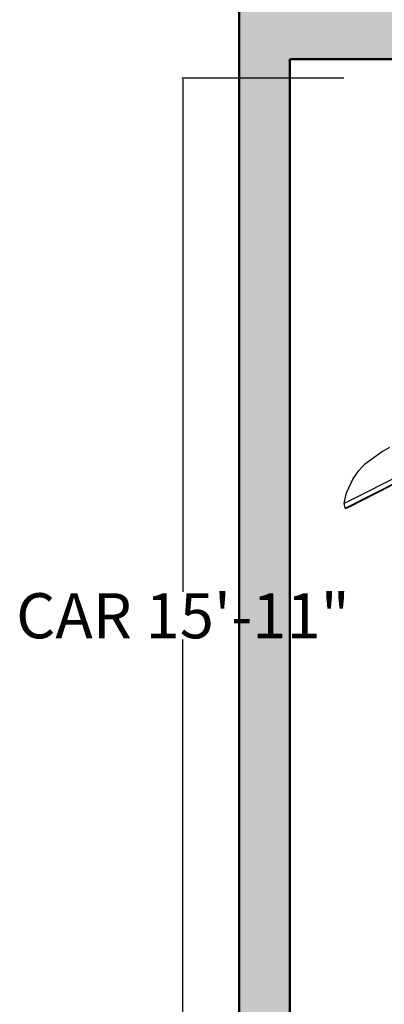
# Model space of a CAD drawing. Units: inches. Extents: x 22042254 to 25404563, y 17568978 to 17626777.
# Tile 25 of 45: x 22179745 to 22179810, y 17626227 to 17626402. Entities that reach past the tile are written whole.
import ezdxf

# ---------------------------------------------------------------- set-up
doc = ezdxf.new("R2010")
doc.units = ezdxf.units.IN
doc.header["$MEASUREMENT"] = 0
for name, color, linetype, lineweight in [('A-ANNO-DIMS', 2, 'Continuous', 18), ('A-SITE-VEHI', 8, 'Continuous', 18), ('A-WALL-PATT', 244, 'Continuous', 13), ('walls', 252, 'Continuous', 50)]:
    doc.layers.add(name, color=color, linetype=linetype, lineweight=lineweight)
doc.layers.add('Edges', color=250, linetype='Continuous')
doc.styles.get("Standard").update_dxf_attribs({"font": 'arial.ttf'})
doc.dimstyles.get("Standard").update_dxf_attribs({"dimtxt": 8, "dimasz": 0.18, "dimexe": 0.18, "dimexo": 0.0625, "dimgap": 0.09, "dimtad": 0, "dimtih": 1, "dimtoh": 1, "dimzin": 0, "dimdsep": 46, "dimlunit": 3, "dimtxsty": 'Standard', "dimcen": 0.09, "dimadec": 0, "dimazin": 0, "dimtfac": 1, "dimtofl": 0, "dimtmove": 0, "dimatfit": 3, "dimfxl": 1, "dimtolj": 1, "dimtzin": 0, "dimarcsym": 0})

# ---------------------------------------------------------------- blocks, each defined once
blk = doc.blocks.new('Nissan Qashqai pl')
at = {"layer": 'Edges'}
for p, q in [((8.8918, 11.0997), (9.0186, 10.8486)), ((9.0333, 10.8597), (8.9232, 11.0779)), ((9.0386, 10.8534), (8.9254, 11.0778)), ((8.9483, 11.0359), (9.0343, 10.8656)), ((8.7908, 11.0322), (8.8066, 11.0041)), ((8.8066, 11.0041), (8.8591, 10.9315)), ((8.8591, 10.9315), (8.8879, 10.9041)), ((8.8885, 10.9037), (8.8879, 10.9041)), ((8.8885, 10.9037), (8.9173, 10.8831)), ((8.9173, 10.8831), (8.9731, 10.8577)), ((9.0186, 10.8486), (8.9731, 10.8577)), ((9.0374, 10.8517), (9.0186, 10.8486)), ((9.0356, 10.8553), (9.0333, 10.8597)), ((9.0343, 10.8656), (9.0347, 10.8648)), ((9.0347, 10.8648), (9.0362, 10.8619)), ((9.0356, 10.8553), (9.0374, 10.8517)), ((9.0362, 10.8619), (9.037, 10.8603)), ((9.0371, 10.8601), (9.037, 10.8603)), ((9.0371, 10.8601), (9.0376, 10.8591)), ((9.0376, 10.8591), (9.0371, 10.8595)), ((9.0386, 10.8534), (9.0374, 10.8517)), ((9.0376, 10.8591), (9.0386, 10.8534))]:
    blk.add_line(p, q, dxfattribs=at)
blk = doc.blocks.new('CAR')
blk.add_blockref('Nissan Qashqai pl', (-9.7433, -11.9151))
blk = doc.blocks.new('*D58')
at = {"layer": 'A-ANNO-DIMS', "color": 0, "lineweight": -2, "transparency": 16777216}
for p, q in [((22179802.34, 17626391.38), (22179773.6, 17626391.38)), ((22179773.78, 17626391.2), (22179773.78, 17626300.19)), ((22179773.78, 17626200.74), (22179773.78, 17626291.74)), ((22179802.34, 17626200.56), (22179773.6, 17626200.56))]:
    blk.add_line(p, q, dxfattribs=at)
at = {"layer": 'A-ANNO-DIMS', "color": 0, "transparency": 16777216}
for points in [[(22179773.75, 17626391.2), (22179773.81, 17626391.2), (22179773.78, 17626391.38)], [(22179773.75, 17626200.74), (22179773.81, 17626200.74), (22179773.78, 17626200.56)]]:
    blk.add_solid(points, dxfattribs=at)
at = {"layer": 'Defpoints', "color": 0, "transparency": 16777216}
for p in [(22179802.4, 17626391.38), (22179773.78, 17626200.56), (22179802.4, 17626200.56)]:
    blk.add_point(p, dxfattribs=at)
at = {"layer": 'A-ANNO-DIMS', "color": 0, "transparency": 16777216, "insert": (22179773.78, 17626295.97), "char_height": 8, "attachment_point": 5}
blk.add_mtext('\\A1;CAR 15\'-11"', dxfattribs=at)

msp = doc.modelspace()

# ---------------------------------------------------------------- hatches: boundary and pattern name
at = {"layer": 'A-WALL-PATT'}
h = msp.add_hatch(color=256, dxfattribs=at)
h.dxf.hatch_style = 1
h.paths.add_polyline_path([(22179792.734, 17626580.28), (22179888.734, 17626580.28), (22179888.734, 17626559.623), (22179893.234, 17626559.623), (22179893.234, 17626580.28), (22179900.438, 17626580.28), (22179900.438, 17626584.78), (22179792.734, 17626584.78), (22179792.734, 17626728.78), (22180134.734, 17626728.78), (22180134.734, 17626584.78), (22180035.602, 17626584.78), (22180004.432, 17626584.78), (22180001.734, 17626584.78), (22180001.734, 17626580.28), (22180134.734, 17626580.28), (22180134.734, 17626404.28), (22180064.487, 17626404.28), (22180064.487, 17626399.78), (22180134.734, 17626399.78), (22180134.734, 17626197.78), (22180143.734, 17626197.78), (22180143.734, 17626737.78), (22179783.734, 17626737.78), (22179783.734, 17626197.78), (22179792.734, 17626197.78), (22179792.734, 17626394.78), (22179936.734, 17626394.78), (22179936.734, 17626383.208), (22179941.234, 17626383.208), (22179941.234, 17626532.28), (22179927.066, 17626532.28), (22179927.066, 17626527.78), (22179928.072, 17626527.78), (22179936.734, 17626527.78), (22179936.734, 17626403.78), (22179792.734, 17626403.78), (22179792.734, 17626527.78), (22179905.094, 17626527.78), (22179905.094, 17626532.28), (22179792.734, 17626532.28)])

# ---------------------------------------------------------------- linework, layer by layer
at = {"layer": 'walls'}
for p, q in [((22179783.734, 17626197.78), (22179783.734, 17626737.78)), ((22179792.734, 17626197.78), (22179792.734, 17626394.78)), ((22179792.734, 17626394.78), (22179936.734, 17626394.78))]:
    msp.add_line(p, q, dxfattribs=at)

# ---------------------------------------------------------------- block references
at = {"layer": 'A-SITE-VEHI', "xscale": 43.56002006885659, "yscale": 43.56002006885659, "zscale": 43.56002006885659, "rotation": 270}
msp.add_blockref('CAR', (22179848.861, 17626284.325), dxfattribs=at)

# ---------------------------------------------------------------- dimensions: what is measured, and where the dimension line sits
at = {"layer": 'A-ANNO-DIMS'}
dim = msp.add_linear_dim(base=(22179773.779, 17626200.559), p1=(22179802.402, 17626391.376), p2=(22179802.402, 17626200.559), angle=270, text='CAR <>', dimstyle='Standard', override={"dimdec": 1, "dimlfac": 1, "dimrnd": 0, "dimzin": 1, "dimdsep": 46, "dimlunit": 4, "dimfrac": 2}, dxfattribs=at)
dim.commit()
dim.dimension.update_dxf_attribs({"geometry": '*D58', "text_midpoint": (22179773.779, 17626295.968)})

doc.saveas('drawing.dxf')
